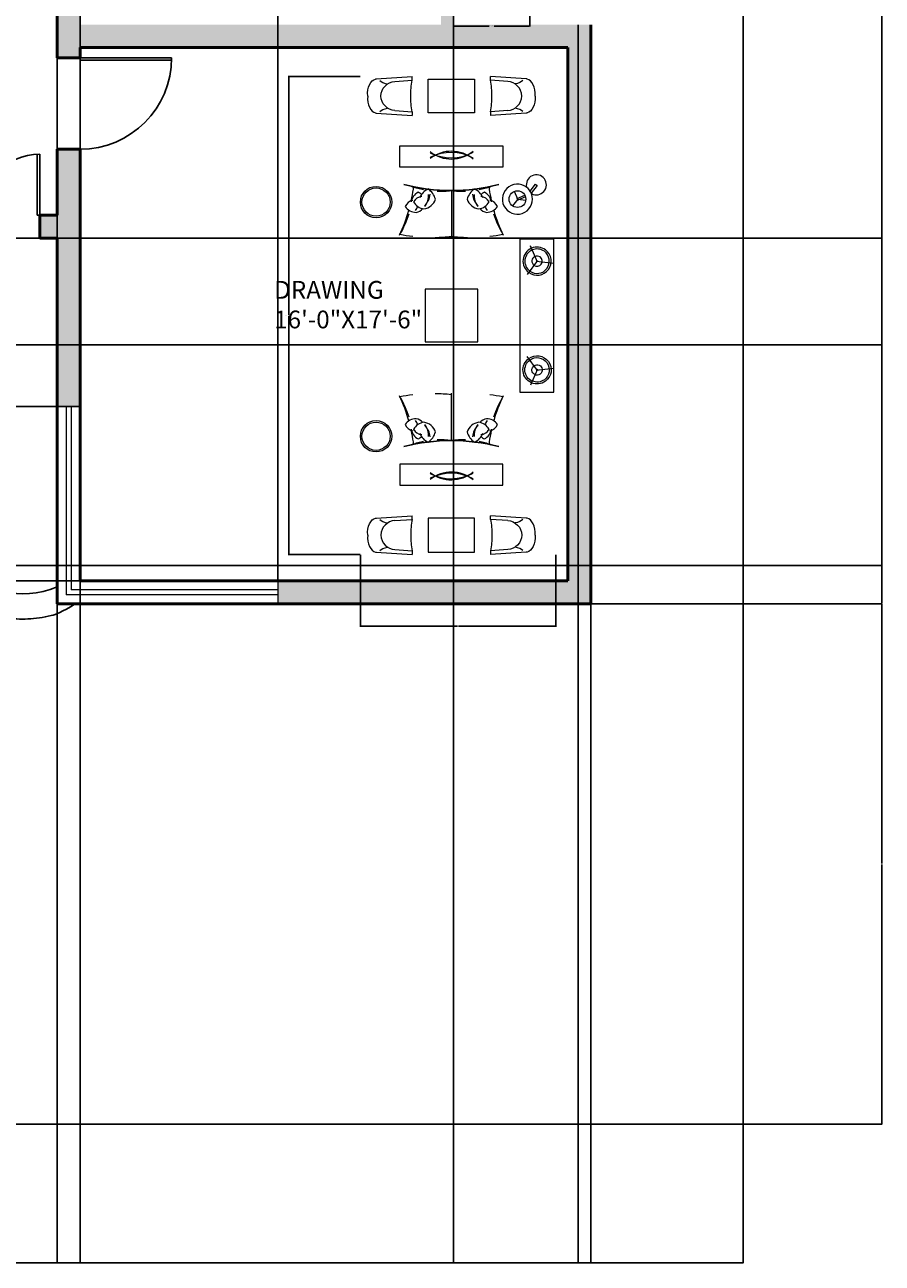
# Model space of a CAD drawing. Units: inches. Extents: x 134045 to 134755, y 144691 to 145880.
# Tile 2 of 6: x 134417 to 134755, y 144691 to 145178. Entities that reach past the tile are written whole.
import ezdxf

# ---------------------------------------------------------------- set-up
doc = ezdxf.new("R2010")
doc.units = ezdxf.units.IN
doc.set_wipeout_variables(frame=1)
for name, color, linetype, lineweight in [('A-ANNO-DIMS', 2, 'Continuous', 18), ('A-AREA-IDEN', 7, 'Continuous', 18), ('A-DOOR', 4, 'Continuous', 25), ('A-FLOR-STEP', 7, 'Continuous', 25), ('A-FURN', 8, 'Continuous', 18), ('A-GLAZ', 4, 'Continuous', 18), ('A-WALL', 7, 'Continuous', 50), ('A-WALL-PATT', 252, 'Continuous', 13), ('C-PROP', 7, 'Continuous', 25)]:
    doc.layers.add(name, color=color, linetype=linetype, lineweight=lineweight)
doc.styles.get("Standard").update_dxf_attribs({"font": 'arial.ttf'})
doc.dimstyles.get("Standard").update_dxf_attribs({"dimtxt": 0.18, "dimasz": 0.18, "dimexe": 0.18, "dimexo": 0.0625, "dimgap": 0.09, "dimtad": 0, "dimtih": 1, "dimtoh": 1, "dimdec": 4, "dimzin": 0, "dimdsep": 46, "dimtxsty": 'Standard', "dimcen": 0.09, "dimadec": 0, "dimazin": 0, "dimtfac": 1, "dimtdec": 4, "dimtofl": 0, "dimtmove": 0, "dimatfit": 3, "dimfxl": 1, "dimtolj": 1, "dimtzin": 0, "dimarcsym": 0})

# ---------------------------------------------------------------- blocks, each defined once
blk = doc.blocks.new('A$C5805318C')
at = {"linetype": 'ByBlock'}
for p, q in [((1718, 2794), (1735, 2817)), ((1718, 2794), (1735, 2817)), ((1829, 2708), (1718, 2794)), ((1829, 2708), (1718, 2794)), ((1735, 2817), (1857, 2723)), ((1735, 2817), (1857, 2723)), ((1945, 2497), (1893, 2622)), ((1945, 2497), (1893, 2622)), ((1919, 2633), (1971, 2508)), ((1919, 2633), (1971, 2508)), ((1955, 2509), (1973, 2636)), ((1955, 2509), (1973, 2636)), ((1955, 2509), (1831, 2459)), ((1955, 2509), (1831, 2459)), ((1971, 2508), (1945, 2497)), ((1971, 2508), (1945, 2497)), ((1955, 2509), (2060, 2427)), ((1955, 2509), (2060, 2427))]:
    blk.add_line(p, q, dxfattribs=at)
for p, q in [((38, 2645), (0, 2075)), ((582, 2645), (620, 2075)), ((7041, 2645), (7003, 2075)), ((7585, 2645), (7623, 2075)), ((77, 2348), (59, 2075)), ((543, 2348), (561, 2075)), ((7080, 2348), (7062, 2075)), ((7545, 2348), (7564, 2075)), ((59, 2075), (0, 2075)), ((561, 2075), (620, 2075)), ((7062, 2075), (7003, 2075)), ((7564, 2075), (7623, 2075)), ((59, 824), (0, 824)), ((38, 254), (0, 824)), ((77, 551), (59, 824)), ((543, 551), (561, 824)), ((561, 824), (620, 824)), ((582, 254), (620, 824)), ((7062, 824), (7003, 824)), ((7041, 254), (7003, 824)), ((7080, 551), (7062, 824)), ((7545, 551), (7564, 824)), ((7564, 824), (7623, 824)), ((7585, 254), (7623, 824))]:
    blk.add_line(p, q)
for centre in [(2002, 250), (5737, 250)]:
    blk.add_circle(centre, 225)
for centre, radius, start, end in [((1727, 2805), 160, 331.0509, 282.9948), ((1955, 2504), 240, 111.272, 142.7738), ((1955, 2504), 240, 111.272, 142.7738)]:
    blk.add_arc(centre, radius, start, end, dxfattribs=at)
for points in [[(310, 2784), (175, 2792), (54, 2736), (40, 2660), (39, 2654), (38, 2649), (38, 2643)], [(310, 2784), (445, 2792), (566, 2736), (580, 2660), (581, 2654), (582, 2649), (582, 2643)], [(7313, 2784), (7178, 2792), (7057, 2736), (7042, 2660), (7041, 2654), (7041, 2649), (7041, 2643)], [(7313, 2784), (7448, 2792), (7569, 2736), (7583, 2660), (7584, 2654), (7585, 2649), (7585, 2643)], [(310, 116), (175, 108), (54, 163), (40, 240), (39, 245), (38, 251), (38, 256)], [(310, 116), (445, 108), (566, 163), (580, 240), (581, 245), (582, 251), (582, 256)], [(7313, 116), (7178, 108), (7057, 163), (7042, 240), (7041, 245), (7041, 251), (7041, 256)], [(7313, 116), (7448, 108), (7569, 163), (7583, 240), (7584, 245), (7585, 251), (7585, 256)]]:
    blk.add_open_spline(points, degree=3, knots=[0, 0, 0, 0, 1, 1, 1, 2, 2, 2, 2])
for points in [[(62, 2590), (86, 2572), (108, 2522), (117, 2466)], [(310, 2572), (188, 2572), (86, 2474), (77, 2348)], [(543, 2348), (534, 2474), (433, 2572), (310, 2572)], [(558, 2590), (535, 2572), (512, 2522), (503, 2466)], [(7065, 2590), (7088, 2572), (7110, 2522), (7119, 2466)], [(7080, 2348), (7089, 2474), (7190, 2572), (7313, 2572)], [(7313, 2572), (7435, 2572), (7537, 2474), (7545, 2348)], [(7561, 2590), (7537, 2572), (7515, 2522), (7506, 2466)], [(310, 2096), (226, 2096), (142, 2089), (59, 2075)], [(561, 2075), (478, 2089), (394, 2096), (310, 2096)], [(7062, 2075), (7145, 2089), (7229, 2096), (7313, 2096)], [(7313, 2096), (7397, 2096), (7481, 2089), (7564, 2075)], [(310, 804), (226, 804), (142, 810), (59, 824)], [(561, 824), (478, 810), (394, 804), (310, 804)], [(7062, 824), (7145, 810), (7229, 804), (7313, 804)], [(7313, 804), (7397, 804), (7481, 810), (7564, 824)], [(62, 310), (86, 327), (108, 378), (117, 434)], [(310, 328), (188, 328), (86, 425), (77, 551)], [(543, 551), (534, 425), (433, 328), (310, 328)], [(558, 310), (535, 327), (512, 378), (503, 434)], [(7065, 310), (7088, 327), (7110, 378), (7119, 434)], [(7080, 551), (7089, 425), (7190, 328), (7313, 328)], [(7313, 328), (7435, 328), (7537, 425), (7545, 551)], [(7561, 310), (7537, 327), (7515, 378), (7506, 434)]]:
    blk.add_open_spline(points, degree=3)
for points in [[(2561, 3114), (2561, 2514), (5061, 2514), (5061, 3114)], [(1474, 600), (1074, 600), (1074, 2300), (1474, 2300)], [(2575, 1450), (2574, 1519), (2572, 1654), (2567, 1805), (2559, 1944), (2549, 2088), (2540, 2188), (2531, 2276), (2527, 2314), (1674, 2200), (1674, 1450), (1674, 699), (2527, 585), (2531, 623), (2540, 712), (2549, 811), (2559, 956), (2567, 1094), (2572, 1246), (2574, 1380)], [(5048, 1450), (5048, 1519), (5051, 1654), (5056, 1805), (5064, 1944), (5074, 2088), (5083, 2188), (5091, 2276), (5096, 2314), (5949, 2200), (5949, 1450), (5949, 699), (5096, 585), (5091, 623), (5083, 712), (5074, 811), (5064, 956), (5056, 1094), (5051, 1246), (5048, 1380)], [(6149, 600), (6549, 600), (6549, 2300), (6149, 2300)], [(610, 1050), (10, 1050), (10, 1850), (610, 1850)], [(3361, 1000), (4261, 1000), (4261, 1900), (3361, 1900)], [(7013, 1050), (7613, 1050), (7613, 1850), (7013, 1850)]]:
    blk.add_wipeout(points, dxfattribs=at)
for p, q in [((2943, 2802), (2974, 3081)), ((2968, 3032), (2974, 3078)), ((4680, 2802), (4649, 3081)), ((4654, 3032), (4649, 3078)), ((2958, 2823), (2701, 2710)), ((2932, 2826), (3159, 2659)), ((4690, 2826), (4464, 2659)), ((4665, 2823), (4922, 2710)), ((2746, 2730), (2704, 2712)), ((3119, 2688), (3156, 2661)), ((4504, 2688), (4467, 2661)), ((4877, 2730), (4919, 2712))]:
    blk.add_line(p, q, dxfattribs=at)
for p, q in [((1817, 1450), (2575, 1450)), ((5805, 1450), (5048, 1450))]:
    blk.add_line(p, q)
for points in [[(2591, 3084), (2591, 2544), (5031, 2544), (5031, 3084)], [(1444, 630), (1104, 630), (1104, 2270), (1444, 2270)], [(6179, 630), (6519, 630), (6519, 2270), (6179, 2270)], [(580, 1080), (40, 1080), (40, 1820), (580, 1820)], [(3391, 1030), (4231, 1030), (4231, 1870), (3391, 1870)], [(7043, 1080), (7583, 1080), (7583, 1820), (7043, 1820)]]:
    blk.add_lwpolyline(points, close=True, dxfattribs=at)
blk.add_circle((1955, 2504), 133, dxfattribs=at)
blk.add_circle((1955, 2504), 133, dxfattribs=at)
for centre in [(2002, 250), (5737, 250)]:
    blk.add_circle(centre, 250)
for centre, radius, start, end in [((1955, 2504), 240, 142.7738, 111.272), ((-1206, 1450), 3024, 345.5057, 14.4943), ((2141, 2032), 169, 113.788, 168.6748), ((1945, 2005), 222, 1.4651, 55.0097), ((1435, 4574), 2546, 285.8776, 295.5087), ((6188, 4574), 2546, 244.4913, 254.1224), ((5678, 2005), 222, 124.9903, 178.5349), ((5482, 2032), 169, 11.3252, 66.212), ((8829, 1450), 3024, 165.5057, 194.4943), ((1785, 2087), 34.6, 193.5328, 287.2771), ((1435, 4574), 2546, 278.134, 282.3755), ((2038, 1878), 217, 100.5196, 152.9581), ((2095, 2106), 282, 207.4684, 220.0792), ((2081, 1906), 169, 119.788, 174.6748), ((1889, 1858), 222, 7.4651, 61.0097), ((1947, 2064), 226, 314.9669, 346.4215), ((5676, 2064), 226, 193.5785, 225.0331), ((5734, 1858), 222, 118.9903, 172.5349), ((5585, 1878), 217, 27.0419, 79.4804), ((5542, 1906), 169, 5.3252, 60.212), ((6188, 4574), 2546, 257.6245, 261.866), ((5528, 2106), 282, 319.9208, 332.5316), ((5838, 2087), 34.6, 252.7229, 346.4672), ((769, 1450), 546, 321.7197, 39.6872), ((1737, 1450), 546, 140.3128, 218.2803), ((564, 1447), 732, 332.7542, 28.6527), ((1942, 1447), 732, 151.3473, 207.2458), ((1996, 1742), 217, 106.5196, 158.9581), ((2028, 1975), 282, 213.4684, 255.3384), ((1885, 1917), 226, 288.0023, 352.4215), ((5738, 1917), 226, 187.5785, 251.9977), ((5595, 1975), 282, 284.6616, 326.5316), ((5627, 1742), 217, 21.0419, 73.4804), ((5885, 1450), 546, 321.7197, 39.6872), ((6854, 1450), 546, 140.3128, 218.2803), ((5681, 1447), 732, 332.7542, 28.6527), ((7058, 1447), 732, 151.3473, 207.2458), ((2028, 924), 282, 104.6616, 146.5316), ((1885, 982), 226, 7.5785, 71.9977), ((5738, 982), 226, 108.0023, 172.4215), ((5595, 924), 282, 33.4684, 75.3384), ((1996, 1158), 217, 201.0419, 253.4804), ((1889, 1041), 222, 298.9903, 352.5349), ((1947, 836), 226, 13.5785, 45.0331), ((5676, 836), 226, 134.9669, 166.4215), ((5734, 1041), 222, 187.4651, 241.0097), ((5627, 1158), 217, 286.5196, 338.9581), ((1785, 813), 34.6, 72.7229, 166.4672), ((1435, -1675), 2546, 77.6245, 81.866), ((2095, 793), 282, 139.9208, 152.5316), ((2038, 1021), 217, 207.0419, 259.4804), ((2081, 993), 169, 185.3252, 240.212), ((2141, 867), 169, 191.3252, 246.212), ((1945, 894), 222, 304.9903, 358.5349), ((5678, 894), 222, 181.4651, 235.0097), ((5482, 867), 169, 293.788, 348.6748), ((5585, 1021), 217, 280.5196, 332.9581), ((5542, 993), 169, 299.788, 354.6748), ((6188, -1675), 2546, 98.134, 102.3755), ((5528, 793), 282, 27.4684, 40.0792), ((5838, 813), 34.6, 13.5328, 107.2771), ((1435, -1675), 2546, 64.4913, 74.1224), ((6188, -1675), 2546, 105.8776, 115.5087)]:
    blk.add_arc(centre, radius, start, end, dxfattribs=at)
for centre, radius, start, end in [((-1206, 1450), 3019, 345.5057, 14.4943), ((1640, 3765), 1733, 288.4757, 300.3241), ((-91, 1753), 2657, 6.7363, 11.1857), ((7714, 1753), 2657, 168.8143, 173.2637), ((5982, 3765), 1733, 239.6759, 251.5243), ((8829, 1450), 3019, 165.5057, 194.4943), ((477, 1627), 1352, 11.274, 19.5243), ((1964, 2245), 282, 292.5627, 307.9208), ((5659, 2245), 282, 232.0792, 247.4373), ((7146, 1627), 1352, 160.4757, 168.726), ((1853, 2068), 282, 275.0195, 316.8895), ((1899, 2095), 282, 266.0508, 307.9208), ((5723, 2095), 282, 232.0792, 273.9492), ((5769, 2068), 282, 223.1105, 264.9805), ((477, 1627), 1352, 352.4802, 2.0119), ((-91, 1753), 2657, 353.4417, 359.0402), ((7146, 1627), 1352, 177.9881, 187.5198), ((477, 1273), 1352, 357.9881, 7.5198), ((-91, 1146), 2657, 0.9598, 6.5583), ((7714, 1146), 2657, 173.4417, 179.0402), ((7146, 1273), 1352, 172.4802, 182.0119), ((477, 1273), 1352, 340.4757, 348.726), ((1853, 831), 282, 43.1105, 84.9805), ((1899, 804), 282, 52.0792, 93.9492), ((5723, 804), 282, 86.0508, 127.9208), ((5769, 831), 282, 95.0195, 136.8895), ((7146, 1273), 1352, 191.274, 199.5243), ((1964, 654), 282, 52.0792, 67.4373), ((-91, 1146), 2657, 348.8143, 353.2637), ((7714, 1146), 2657, 186.7363, 191.1857), ((5659, 654), 282, 112.5627, 127.9208), ((1640, -865), 1733, 59.6759, 71.5243), ((5982, -865), 1733, 108.4757, 120.3241)]:
    blk.add_arc(centre, radius, start, end)
for major_axis, start_param, end_param in [((-159, 159), 3.292387, 6.433979), ((-138, 138), 3.292387, 6.433979), ((-159, 159), 0.150794, 3.292387), ((-138, 138), 0.150794, 3.292387), ((-58.4, 58.4), 0.150794, 3.292387), ((-58.4, 58.4), 3.292387, 6.433979)]:
    blk.add_ellipse((2944, 2817), major_axis=major_axis, ratio=1, start_param=start_param, end_param=end_param, dxfattribs=at)
at = {"linetype": 'ByBlock', "extrusion": (0, 0, -1)}
for major_axis, start_param, end_param in [((159, 159), 3.292387, 6.433979), ((138, 138), 3.292387, 6.433979), ((159, 159), 0.150794, 3.292387), ((138, 138), 0.150794, 3.292387), ((-58.4, 58.4), 4.863183, 8.004776), ((-58.4, 58.4), 1.72159, 4.863183)]:
    blk.add_ellipse((4678, 2817), major_axis=major_axis, ratio=1, start_param=start_param, end_param=end_param, dxfattribs=at)
blk = doc.blocks.new('DOOR-SWING-36IN')
for p, q in [((0, 1), (35.99, 1)), ((0, 0), (0, 1)), ((0, 0), (36, 0))]:
    blk.add_line(p, q)
blk.add_arc((0, 0), 36, 0, 90)
blk = doc.blocks.new('DOOR-SWING-24IN')
for p, q in [((0, 0), (0, 24)), ((1, 0), (1, 23.98)), ((1, 0), (0, 0))]:
    blk.add_line(p, q)
blk.add_arc((0, 0), 24, 0, 90)
blk = doc.blocks.new('*D22')
at = {"layer": 'A-ANNO-DIMS', "color": 0, "lineweight": -2, "transparency": 16777216}
for p, q in [((134586.1, 145182.31), (134586.1, 145177.7)), ((134586.28, 145177.88), (134600.17, 145177.88)), ((134615.92, 145177.88), (134602.04, 145177.88)), ((134616.1, 145182.31), (134616.1, 145177.7))]:
    blk.add_line(p, q, dxfattribs=at)
at = {"layer": 'A-ANNO-DIMS', "color": 0, "transparency": 16777216}
for points in [[(134586.28, 145177.91), (134586.28, 145177.85), (134586.1, 145177.88)], [(134615.92, 145177.91), (134615.92, 145177.85), (134616.1, 145177.88)]]:
    blk.add_solid(points, dxfattribs=at)
at = {"layer": 'Defpoints', "color": 0, "transparency": 16777216}
for p in [(134586.1, 145182.38), (134616.1, 145182.38), (134616.1, 145177.88)]:
    blk.add_point(p, dxfattribs=at)
at = {"layer": 'A-ANNO-DIMS', "color": 0, "transparency": 16777216, "insert": (134601.1, 145177.88), "char_height": 0.18, "attachment_point": 5}
blk.add_mtext('\\A1;DOOR 30 TYP.', dxfattribs=at)
blk = doc.blocks.new('*D38')
at = {"layer": 'A-ANNO-DIMS', "color": 0, "lineweight": -2, "transparency": 16777216}
for p, q in [((134549.36, 145157.98), (134521.01, 145157.98)), ((134521.19, 145157.8), (134521.19, 145064.04)), ((134521.19, 144969.92), (134521.19, 145063.67)), ((134549.36, 144969.74), (134521.01, 144969.74))]:
    blk.add_line(p, q, dxfattribs=at)
at = {"layer": 'A-ANNO-DIMS', "color": 0, "transparency": 16777216}
for points in [[(134521.16, 145157.8), (134521.22, 145157.8), (134521.19, 145157.98)], [(134521.16, 144969.92), (134521.22, 144969.92), (134521.19, 144969.74)]]:
    blk.add_solid(points, dxfattribs=at)
at = {"layer": 'Defpoints', "color": 0, "transparency": 16777216}
for p in [(134549.42, 145157.98), (134521.19, 144969.74), (134549.42, 144969.74)]:
    blk.add_point(p, dxfattribs=at)
at = {"layer": 'A-ANNO-DIMS', "color": 0, "transparency": 16777216, "insert": (134521.19, 145063.86), "char_height": 0.18, "attachment_point": 5}
blk.add_mtext('\\A1;SEATING GROUP 188', dxfattribs=at)
blk = doc.blocks.new('*D39')
at = {"layer": 'A-ANNO-DIMS', "color": 0, "lineweight": -2, "transparency": 16777216}
for p, q in [((134549.42, 144969.68), (134549.42, 144941.33)), ((134626.31, 144969.68), (134626.31, 144941.33)), ((134549.6, 144941.51), (134587.65, 144941.51)), ((134626.13, 144941.51), (134588.09, 144941.51))]:
    blk.add_line(p, q, dxfattribs=at)
at = {"layer": 'A-ANNO-DIMS', "color": 0, "transparency": 16777216}
for points in [[(134549.6, 144941.54), (134549.6, 144941.48), (134549.42, 144941.51)], [(134626.13, 144941.54), (134626.13, 144941.48), (134626.31, 144941.51)]]:
    blk.add_solid(points, dxfattribs=at)
at = {"layer": 'Defpoints', "color": 0, "transparency": 16777216}
for p in [(134549.42, 144969.74), (134626.31, 144969.74), (134626.31, 144941.51)]:
    blk.add_point(p, dxfattribs=at)
at = {"layer": 'A-ANNO-DIMS', "color": 0, "transparency": 16777216, "insert": (134587.87, 144941.51), "char_height": 0.18, "attachment_point": 5}
blk.add_mtext('\\A1;77', dxfattribs=at)
blk = doc.blocks.new('*D46')
at = {"layer": 'A-ANNO-DIMS', "color": 0, "lineweight": -2, "transparency": 16777216}
for p, q in [((134100.1, 144745.31), (134100.1, 144690.65)), ((134700.1, 144745.31), (134700.1, 144690.65)), ((134100.28, 144690.83), (134399.81, 144690.83)), ((134699.92, 144690.83), (134400.39, 144690.83))]:
    blk.add_line(p, q, dxfattribs=at)
at = {"layer": 'A-ANNO-DIMS', "color": 0, "transparency": 16777216}
for points in [[(134100.28, 144690.86), (134100.28, 144690.8), (134100.1, 144690.83)], [(134699.92, 144690.86), (134699.92, 144690.8), (134700.1, 144690.83)]]:
    blk.add_solid(points, dxfattribs=at)
at = {"layer": 'Defpoints', "color": 0, "transparency": 16777216}
for p in [(134100.1, 144745.38), (134700.1, 144745.38), (134700.1, 144690.83)]:
    blk.add_point(p, dxfattribs=at)
at = {"layer": 'A-ANNO-DIMS', "color": 0, "transparency": 16777216, "insert": (134400.1, 144690.83), "char_height": 0.18, "attachment_point": 5}
blk.add_mtext('\\A1;600', dxfattribs=at)
blk = doc.blocks.new('*D49')
at = {"layer": 'A-ANNO-DIMS', "color": 0, "lineweight": -2, "transparency": 16777216}
for p, q in [((134640.17, 145765.38), (134754.83, 145765.38)), ((134754.65, 145765.2), (134754.65, 145358.06)), ((134754.65, 144950.56), (134754.65, 145357.69)), ((134640.17, 144950.38), (134754.83, 144950.38))]:
    blk.add_line(p, q, dxfattribs=at)
at = {"layer": 'A-ANNO-DIMS', "color": 0, "transparency": 16777216}
for points in [[(134754.62, 145765.2), (134754.68, 145765.2), (134754.65, 145765.38)], [(134754.62, 144950.56), (134754.68, 144950.56), (134754.65, 144950.38)]]:
    blk.add_solid(points, dxfattribs=at)
at = {"layer": 'Defpoints', "color": 0, "transparency": 16777216}
for p in [(134640.1, 145765.38), (134754.65, 145765.38), (134640.1, 144950.38)]:
    blk.add_point(p, dxfattribs=at)
at = {"layer": 'A-ANNO-DIMS', "color": 0, "transparency": 16777216, "insert": (134754.65, 145357.88), "char_height": 0.18, "attachment_point": 5}
blk.add_mtext('\\A1;815', dxfattribs=at)
blk = doc.blocks.new('*D53')
at = {"layer": 'A-ANNO-DIMS', "color": 0, "lineweight": -2, "transparency": 16777216}
for p, q in [((134640.17, 144950.38), (134754.83, 144950.38)), ((134754.65, 144950.2), (134754.65, 144848.06)), ((134754.65, 144745.56), (134754.65, 144847.69)), ((134700.17, 144745.38), (134754.83, 144745.38))]:
    blk.add_line(p, q, dxfattribs=at)
at = {"layer": 'A-ANNO-DIMS', "color": 0, "transparency": 16777216}
for points in [[(134754.62, 144950.2), (134754.68, 144950.2), (134754.65, 144950.38)], [(134754.62, 144745.56), (134754.68, 144745.56), (134754.65, 144745.38)]]:
    blk.add_solid(points, dxfattribs=at)
at = {"layer": 'Defpoints', "color": 0, "transparency": 16777216}
for p in [(134640.1, 144950.38), (134700.1, 144745.38), (134754.65, 144745.38)]:
    blk.add_point(p, dxfattribs=at)
at = {"layer": 'A-ANNO-DIMS', "color": 0, "transparency": 16777216, "insert": (134754.65, 144847.88), "char_height": 0.18, "attachment_point": 5}
blk.add_mtext('\\A1;205', dxfattribs=at)
blk = doc.blocks.new('*D56')
at = {"layer": 'A-ANNO-DIMS', "color": 0, "lineweight": -2, "transparency": 16777216}
for p, q in [((134298.17, 145094.38), (134754.83, 145094.38)), ((134754.65, 145094.2), (134754.65, 145073.56)), ((134754.65, 145052.56), (134754.65, 145073.19)), ((134298.17, 145052.38), (134754.83, 145052.38))]:
    blk.add_line(p, q, dxfattribs=at)
at = {"layer": 'A-ANNO-DIMS', "color": 0, "transparency": 16777216}
for points in [[(134754.62, 145094.2), (134754.68, 145094.2), (134754.65, 145094.38)], [(134754.62, 145052.56), (134754.68, 145052.56), (134754.65, 145052.38)]]:
    blk.add_solid(points, dxfattribs=at)
at = {"layer": 'Defpoints', "color": 0, "transparency": 16777216}
for p in [(134298.1, 145094.38), (134754.65, 145094.38), (134298.1, 145052.38)]:
    blk.add_point(p, dxfattribs=at)
at = {"layer": 'A-ANNO-DIMS', "color": 0, "transparency": 16777216, "insert": (134754.65, 145073.38), "char_height": 0.18, "attachment_point": 5}
blk.add_mtext('\\A1;42', dxfattribs=at)
blk = doc.blocks.new('*D62')
at = {"layer": 'A-ANNO-DIMS', "color": 0, "lineweight": -2, "transparency": 16777216}
for p, q in [((134586.1, 145178.31), (134586.1, 144690.65)), ((134635.1, 145178.31), (134635.1, 144690.65)), ((134586.28, 144690.83), (134610.38, 144690.83)), ((134634.92, 144690.83), (134610.83, 144690.83))]:
    blk.add_line(p, q, dxfattribs=at)
at = {"layer": 'A-ANNO-DIMS', "color": 0, "transparency": 16777216}
for points in [[(134586.28, 144690.86), (134586.28, 144690.8), (134586.1, 144690.83)], [(134634.92, 144690.86), (134634.92, 144690.8), (134635.1, 144690.83)]]:
    blk.add_solid(points, dxfattribs=at)
at = {"layer": 'Defpoints', "color": 0, "transparency": 16777216}
for p in [(134586.1, 145178.38), (134635.1, 145178.38), (134635.1, 144690.83)]:
    blk.add_point(p, dxfattribs=at)
at = {"layer": 'A-ANNO-DIMS', "color": 0, "transparency": 16777216, "insert": (134610.6, 144690.83), "char_height": 0.18, "attachment_point": 5}
blk.add_mtext('\\A1;49', dxfattribs=at)
blk = doc.blocks.new('*D63')
at = {"layer": 'A-ANNO-DIMS', "color": 0, "lineweight": -2, "transparency": 16777216}
for p, q in [((134635.1, 145178.31), (134635.1, 144690.65)), ((134640.1, 145178.31), (134640.1, 144690.65)), ((134635.28, 144690.83), (134637.45, 144690.83)), ((134639.92, 144690.83), (134637.75, 144690.83))]:
    blk.add_line(p, q, dxfattribs=at)
at = {"layer": 'A-ANNO-DIMS', "color": 0, "transparency": 16777216}
for points in [[(134635.28, 144690.86), (134635.28, 144690.8), (134635.1, 144690.83)], [(134639.92, 144690.86), (134639.92, 144690.8), (134640.1, 144690.83)]]:
    blk.add_solid(points, dxfattribs=at)
at = {"layer": 'Defpoints', "color": 0, "transparency": 16777216}
for p in [(134635.1, 145178.38), (134640.1, 145178.38), (134640.1, 144690.83)]:
    blk.add_point(p, dxfattribs=at)
at = {"layer": 'A-ANNO-DIMS', "color": 0, "transparency": 16777216, "insert": (134637.6, 144690.83), "char_height": 0.18, "attachment_point": 5}
blk.add_mtext('\\A1;5', dxfattribs=at)
blk = doc.blocks.new('*D64')
at = {"layer": 'A-ANNO-DIMS', "color": 0, "lineweight": -2, "transparency": 16777216}
for p, q in [((134430.1, 145182.31), (134430.1, 144690.65)), ((134439.1, 145178.31), (134439.1, 144690.65)), ((134430.28, 144690.83), (134434.45, 144690.83)), ((134438.92, 144690.83), (134434.75, 144690.83))]:
    blk.add_line(p, q, dxfattribs=at)
at = {"layer": 'A-ANNO-DIMS', "color": 0, "transparency": 16777216}
for points in [[(134430.28, 144690.86), (134430.28, 144690.8), (134430.1, 144690.83)], [(134438.92, 144690.86), (134438.92, 144690.8), (134439.1, 144690.83)]]:
    blk.add_solid(points, dxfattribs=at)
at = {"layer": 'Defpoints', "color": 0, "transparency": 16777216}
for p in [(134430.1, 145182.38), (134439.1, 145178.38), (134439.1, 144690.83)]:
    blk.add_point(p, dxfattribs=at)
at = {"layer": 'A-ANNO-DIMS', "color": 0, "transparency": 16777216, "insert": (134434.6, 144690.83), "char_height": 0.18, "attachment_point": 5}
blk.add_mtext('\\A1;9', dxfattribs=at)
blk = doc.blocks.new('*D65')
at = {"layer": 'A-ANNO-DIMS', "color": 0, "lineweight": -2, "transparency": 16777216}
for p, q in [((134365.99, 144965.38), (134754.83, 144965.38)), ((134754.65, 144965.2), (134754.65, 144958.06)), ((134754.65, 144950.56), (134754.65, 144957.69)), ((134430.17, 144950.38), (134754.83, 144950.38))]:
    blk.add_line(p, q, dxfattribs=at)
at = {"layer": 'A-ANNO-DIMS', "color": 0, "transparency": 16777216}
for points in [[(134754.62, 144965.2), (134754.68, 144965.2), (134754.65, 144965.38)], [(134754.62, 144950.56), (134754.68, 144950.56), (134754.65, 144950.38)]]:
    blk.add_solid(points, dxfattribs=at)
at = {"layer": 'Defpoints', "color": 0, "transparency": 16777216}
for p in [(134365.92, 144965.38), (134754.65, 144965.38), (134430.1, 144950.38)]:
    blk.add_point(p, dxfattribs=at)
at = {"layer": 'A-ANNO-DIMS', "color": 0, "transparency": 16777216, "insert": (134754.65, 144957.88), "char_height": 0.18, "attachment_point": 5}
blk.add_mtext('\\A1;15', dxfattribs=at)
blk = doc.blocks.new('*D66')
at = {"layer": 'A-ANNO-DIMS', "color": 0, "lineweight": -2, "transparency": 16777216}
for p, q in [((134439.1, 144959.44), (134439.1, 145880.11)), ((134516.9, 144959.44), (134516.9, 145880.11)), ((134439.28, 145879.93), (134477.68, 145879.93)), ((134516.72, 145879.93), (134478.32, 145879.93))]:
    blk.add_line(p, q, dxfattribs=at)
at = {"layer": 'A-ANNO-DIMS', "color": 0, "transparency": 16777216}
for points in [[(134439.28, 145879.96), (134439.28, 145879.9), (134439.1, 145879.93)], [(134516.72, 145879.96), (134516.72, 145879.9), (134516.9, 145879.93)]]:
    blk.add_solid(points, dxfattribs=at)
at = {"layer": 'Defpoints', "color": 0, "transparency": 16777216}
for p in [(134516.9, 145879.93), (134439.1, 144959.38), (134516.9, 144959.38)]:
    blk.add_point(p, dxfattribs=at)
at = {"layer": 'A-ANNO-DIMS', "color": 0, "transparency": 16777216, "insert": (134478, 145879.93), "char_height": 0.18, "attachment_point": 5}
blk.add_mtext('\\A1;77.8', dxfattribs=at)
blk = doc.blocks.new('*D67')
at = {"layer": 'A-ANNO-DIMS', "color": 0, "lineweight": -2, "transparency": 16777216}
for p, q in [((134439.04, 145028.04), (134045.37, 145028.04)), ((134045.55, 145027.86), (134045.55, 144993.89)), ((134045.55, 144959.56), (134045.55, 144993.53)), ((134439.04, 144959.38), (134045.37, 144959.38))]:
    blk.add_line(p, q, dxfattribs=at)
at = {"layer": 'A-ANNO-DIMS', "color": 0, "transparency": 16777216}
for points in [[(134045.52, 145027.86), (134045.58, 145027.86), (134045.55, 145028.04)], [(134045.52, 144959.56), (134045.58, 144959.56), (134045.55, 144959.38)]]:
    blk.add_solid(points, dxfattribs=at)
at = {"layer": 'Defpoints', "color": 0, "transparency": 16777216}
for p in [(134045.55, 145028.04), (134439.1, 145028.04), (134439.1, 144959.38)]:
    blk.add_point(p, dxfattribs=at)
at = {"layer": 'A-ANNO-DIMS', "color": 0, "transparency": 16777216, "insert": (134045.55, 144993.71), "char_height": 0.18, "attachment_point": 5}
blk.add_mtext('\\A1;68.66', dxfattribs=at)

msp = doc.modelspace()

# ---------------------------------------------------------------- hatches: boundary and pattern name
at = {"layer": 'A-WALL-PATT'}
h = msp.add_hatch(color=256, dxfattribs=at)
h.dxf.hatch_style = 1
h.paths.add_polyline_path([(134640.1037, 145178.3753), (134586.1037, 145178.3753), (134586.1037, 145182.3753), (134581.1037, 145182.3753), (134581.1037, 145178.3753), (134439.1037, 145178.3753), (134439.1037, 145182.3753), (134430.1037, 145182.3753), (134430.1037, 145165.3753), (134439.1037, 145165.3753), (134439.1037, 145169.3753), (134631.1037, 145169.3753), (134631.1037, 144959.3753), (134516.8973, 144959.3753), (134516.8973, 144950.3753), (134640.1037, 144950.3753)])
h.paths.add_polyline_path([(134439.1037, 145129.3753), (134430.1037, 145129.3753), (134430.1037, 145103.3753), (134423.1948, 145103.3753), (134423.1948, 145094.3753), (134430.1037, 145094.3753), (134430.1037, 145028.0394), (134439.1037, 145028.0394)])

# ---------------------------------------------------------------- linework, layer by layer
at = {"layer": 'A-FLOR-STEP'}
msp.add_open_spline([(134430.1037, 144957.0094), (134399.3308, 144944.8123), (134380.3033, 144978.1647), (134367.1819, 144974.3753)], degree=3, dxfattribs=at)
msp.add_open_spline([(134437.1757, 144950.3753), (134431.726, 144946.8956), (134429.6738, 144946.2317), (134424.5415, 144944.9303), (134421.4861, 144944.4905), (134415.5549, 144944.2239), (134412.6813, 144944.3964), (134407.1936, 144945.2148), (134404.5797, 144945.8591), (134399.6343, 144947.459), (134397.3016, 144948.4141), (134392.9017, 144950.4905), (134390.8335, 144951.612), (134386.3854, 144954.2214), (134384.0816, 144955.7235), (134379.8453, 144958.5591), (134377.9107, 144959.8932), (134375.0049, 144961.8012), (134373.9221, 144962.4818), (134372.0202, 144963.5793), (134371.2004, 144963.9937), (134370.0661, 144964.4771), (134369.6889, 144964.5945), (134365.9246, 144965.3753)], degree=3, knots=[0, 0, 0, 0, 0.49462993, 0.49462993, 1.24835968, 1.24835968, 2.00208942, 2.00208942, 2.75581917, 2.75581917, 3.50954892, 3.50954892, 4.26327867, 4.26327867, 5.23068651, 5.23068651, 6.19809434, 6.19809434, 6.86222056, 6.86222056, 7.52634677, 7.52634677, 8.06757639, 8.06757639, 8.06757639, 8.06757639], dxfattribs=at)
at = {"layer": 'A-GLAZ'}
for p, q in [((134430.1037, 145028.0394), (134439.1037, 145028.0394)), ((134433.6037, 145028.0394), (134433.6037, 144953.8753)), ((134435.6037, 145028.0394), (134435.6037, 144955.8753)), ((134516.8973, 144959.3753), (134516.8973, 144950.3753)), ((134516.8973, 144953.8753), (134433.6037, 144953.8753)), ((134516.8973, 144955.8753), (134435.6037, 144955.8753))]:
    msp.add_line(p, q, dxfattribs=at)
at = {"layer": 'A-WALL'}
for p, q in [((134430.1037, 145165.3753), (134430.1037, 145182.3753)), ((134640.1037, 145178.3753), (134640.1037, 144950.3753)), ((134439.1037, 145169.3753), (134631.1037, 145169.3753)), ((134439.1037, 145169.3753), (134439.1037, 145165.3753)), ((134631.1037, 145169.3753), (134631.1037, 144959.3753)), ((134430.1037, 145165.3753), (134439.1037, 145165.3753)), ((134430.1037, 145103.3753), (134430.1037, 145129.3753)), ((134430.1037, 145129.3753), (134439.1037, 145129.3753)), ((134439.1037, 145129.3753), (134439.1037, 144959.3753)), ((134423.1948, 145103.3753), (134423.1948, 145094.3753)), ((134423.1948, 145103.3753), (134430.1037, 145103.3753)), ((134423.1948, 145094.3753), (134430.1037, 145094.3753)), ((134430.1037, 144950.3753), (134430.1037, 145094.3753)), ((134439.1037, 144959.3753), (134631.1037, 144959.3753)), ((134430.1037, 144950.3753), (134640.1037, 144950.3753))]:
    msp.add_line(p, q, dxfattribs=at)
at = {"layer": 'C-PROP'}
for p, q in [((134700.1037, 145825.3753), (134700.1037, 144745.3753)), ((134700.1037, 144745.3753), (134100.1037, 144745.3753))]:
    msp.add_line(p, q, dxfattribs=at)

# ---------------------------------------------------------------- block references
at = {"layer": 'A-DOOR', "extrusion": (0, 0, -1), "zscale": -1, "rotation": 180}
msp.add_blockref('DOOR-SWING-36IN', (-134439.104, 145165.3757), dxfattribs=at)
at = {"layer": 'A-DOOR', "extrusion": (0, 0, -1), "zscale": -1}
msp.add_blockref('DOOR-SWING-24IN', (-134423.1946, 145103.375), dxfattribs=at)

# ---------------------------------------------------------------- texts
at = {"layer": 'A-AREA-IDEN', "insert": (134515.4596, 145077.4839), "char_height": 7, "attachment_point": 1}
msp.add_mtext_dynamic_manual_height_columns('DRAWING\\P16\'-0"X17\'-6"', width=58.458321, gutter_width=12.5, heights=[0], dxfattribs=at)

# ---------------------------------------------------------------- dimensions: what is measured, and where the dimension line sits
at = {"layer": 'A-ANNO-DIMS'}
for base, p1, p2, override, picture, middle in [((134516.8973, 145879.9253), (134439.1037, 144959.3753), (134516.8973, 144959.3753), {"dimdec": 1, "dimlfac": 1, "dimrnd": 0, "dimzin": 0, "dimdsep": 46, "dimlunit": 2}, '*D66', (134478.0005, 145879.9253)), ((134439.1037, 144690.8253), (134430.1037, 145182.3753), (134439.1037, 145178.3753), {"dimdec": 0, "dimlfac": 1, "dimrnd": 0, "dimzin": 0, "dimdsep": 46, "dimlunit": 2}, '*D64', (134434.6037, 144690.8253)), ((134640.1037, 144690.8253), (134635.1037, 145178.3753), (134640.1037, 145178.3753), {"dimdec": 0, "dimlfac": 1, "dimrnd": 0, "dimzin": 0, "dimdsep": 46, "dimlunit": 2}, '*D63', (134637.6037, 144690.8253)), ((134700.1037, 144690.8253), (134100.1037, 144745.3753), (134700.1037, 144745.3753), {"dimdec": 0, "dimlfac": 1, "dimrnd": 0, "dimzin": 0, "dimdsep": 46, "dimlunit": 2}, '*D46', (134400.1037, 144690.8253))]:
    dim = msp.add_linear_dim(base=base, p1=p1, p2=p2, dimstyle='Standard', override=override, dxfattribs=at)
    dim.commit()
    dim.dimension.update_dxf_attribs({"geometry": picture, "text_midpoint": middle})
for base, p1, p2, override, picture, middle in [((134754.6537, 145765.3753), (134640.1037, 144950.3753), (134640.1037, 145765.3753), {"dimdec": 0, "dimlfac": 1, "dimrnd": 0, "dimzin": 0, "dimdsep": 46, "dimlunit": 2}, '*D49', (134754.6537, 145357.8753)), ((134045.5537, 145028.0394), (134439.1037, 144959.3753), (134439.1037, 145028.0394), {"dimdec": 2, "dimlfac": 1, "dimrnd": 0, "dimzin": 0, "dimdsep": 46, "dimlunit": 2}, '*D67', (134045.5537, 144993.7074)), ((134754.6537, 144965.3753), (134430.1037, 144950.3753), (134365.9246, 144965.3753), {"dimdec": 0, "dimlfac": 1, "dimrnd": 0, "dimzin": 0, "dimdsep": 46, "dimlunit": 2}, '*D65', (134754.6537, 144957.8753)), ((134754.6537, 144745.3753), (134640.1037, 144950.3753), (134700.1037, 144745.3753), {"dimdec": 0, "dimlfac": 1, "dimrnd": 0, "dimzin": 0, "dimdsep": 46, "dimlunit": 2}, '*D53', (134754.6537, 144847.8753))]:
    dim = msp.add_linear_dim(base=base, p1=p1, p2=p2, angle=90, dimstyle='Standard', override=override, dxfattribs=at)
    dim.commit()
    dim.dimension.update_dxf_attribs({"geometry": picture, "text_midpoint": middle})
dim = msp.add_linear_dim(base=(134616.1037, 145177.8753), p1=(134586.1037, 145182.3753), p2=(134616.1037, 145182.3753), text='DOOR <> TYP.', dimstyle='Standard', override={"dimdec": 0, "dimlfac": 1, "dimrnd": 0, "dimzin": 0, "dimdsep": 46, "dimlunit": 2}, dxfattribs=at)
dim.commit()
dim.dimension.update_dxf_attribs({"geometry": '*D22', "text_midpoint": (134601.1037, 145177.8753)})

# ---------------------------------------------------------------- next in the draw order: block references
at = {"layer": 'A-FURN', "xscale": 0.0246935795389962, "yscale": 0.0246935795389962, "zscale": 0.0246935795389962, "rotation": 270}
msp.add_blockref('A$C5805318C', (134549.4215, 145157.9753), dxfattribs=at)

# ---------------------------------------------------------------- next in the draw order: dimensions: what is measured, and where the dimension line sits
at = {"layer": 'A-ANNO-DIMS'}
for base, p1, p2, picture, middle in [((134635.1037, 144690.8253), (134586.1037, 145178.3753), (134635.1037, 145178.3753), '*D62', (134610.6037, 144690.8253)), ((134626.3139, 144941.5053), (134549.4215, 144969.7405), (134626.3139, 144969.7405), '*D39', (134587.8677, 144941.5053))]:
    dim = msp.add_linear_dim(base=base, p1=p1, p2=p2, dimstyle='Standard', override={"dimdec": 0, "dimlfac": 1, "dimrnd": 0, "dimzin": 0, "dimdsep": 46, "dimlunit": 2}, dxfattribs=at)
    dim.commit()
    dim.dimension.update_dxf_attribs({"geometry": picture, "text_midpoint": middle})
dim = msp.add_linear_dim(base=(134521.1863, 144969.7405), p1=(134549.4215, 145157.9753), p2=(134549.4215, 144969.7405), angle=270, text='SEATING GROUP <>', dimstyle='Standard', override={"dimdec": 0, "dimlfac": 1, "dimrnd": 0, "dimzin": 0, "dimdsep": 46, "dimlunit": 2}, dxfattribs=at)
dim.commit()
dim.dimension.update_dxf_attribs({"geometry": '*D38', "text_midpoint": (134521.1863, 145063.8579)})
dim = msp.add_linear_dim(base=(134754.6537, 145094.3753), p1=(134298.1037, 145052.3753), p2=(134298.1037, 145094.3753), angle=90, dimstyle='Standard', override={"dimdec": 0, "dimlfac": 1, "dimrnd": 0, "dimzin": 0, "dimdsep": 46, "dimlunit": 2}, dxfattribs=at)
dim.commit()
dim.dimension.update_dxf_attribs({"geometry": '*D56', "text_midpoint": (134754.6537, 145073.3753)})

doc.saveas('drawing.dxf')
